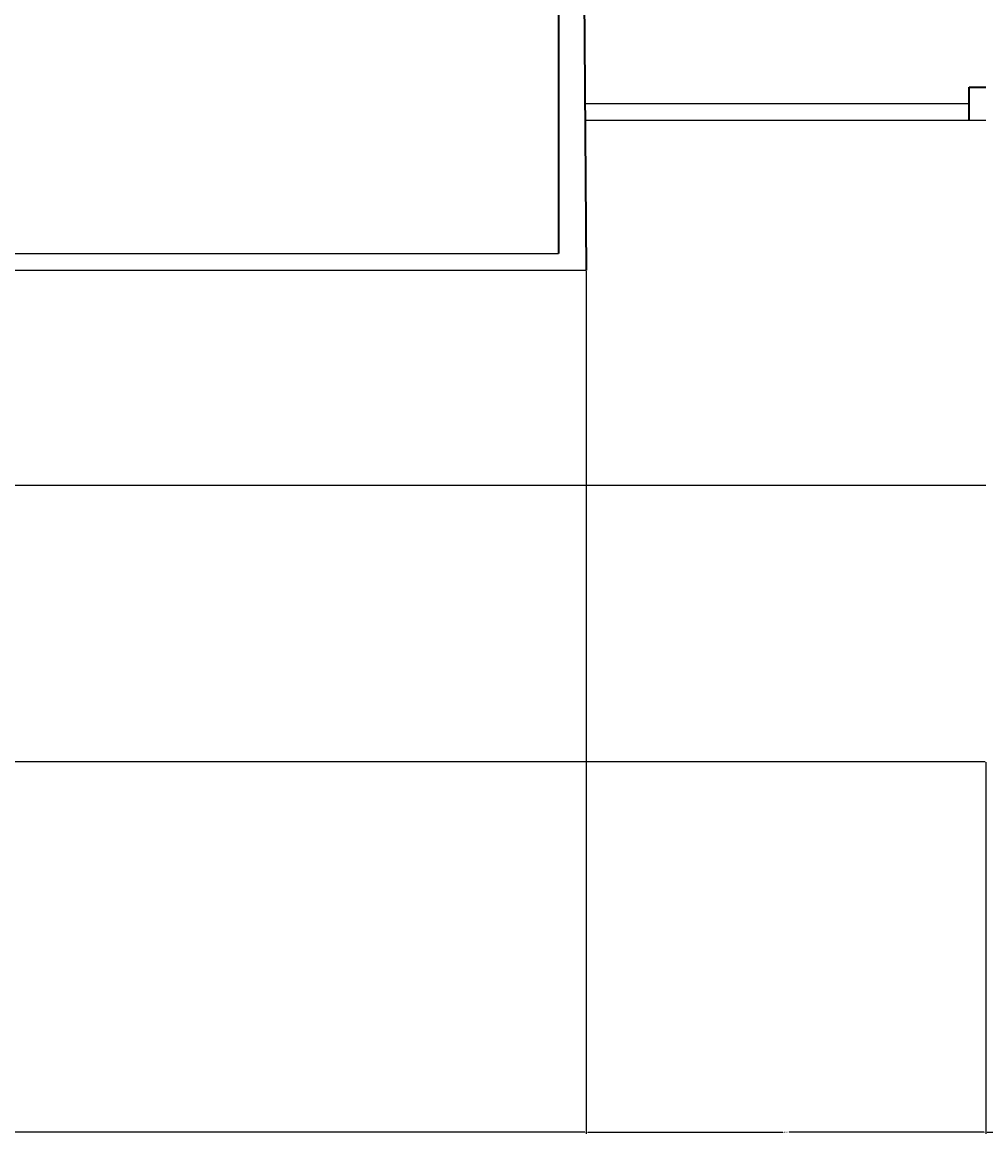
# Model space of a CAD drawing. Units: inches. Extents: x 1002 to 1561, y 1016 to 1994.
# Tile 2 of 8: x 1166 to 1282, y 1016 to 1149. Entities that reach past the tile are written whole.
import ezdxf

# ---------------------------------------------------------------- set-up
doc = ezdxf.new("R2010")
doc.units = ezdxf.units.IN
doc.header["$MEASUREMENT"] = 0
doc.layers.add('A-ANNO-DIMS', color=2, linetype='Continuous', lineweight=18)
doc.layers.add('A-WALL', color=7, linetype='Continuous', lineweight=35)
doc.layers.add('A-FLOR-EDGE', color=217, linetype='Continuous', lineweight=25, true_color=0x93278f)
doc.styles.get("Standard").update_dxf_attribs({"font": 'arial.ttf'})
doc.dimstyles.get("Standard").update_dxf_attribs({"dimtxt": 0.18, "dimasz": 0.18, "dimexe": 0.18, "dimexo": 0.0625, "dimgap": 0.09, "dimtad": 0, "dimtih": 1, "dimtoh": 1, "dimdec": 4, "dimzin": 0, "dimdsep": 46, "dimtxsty": 'Standard', "dimcen": 0.09, "dimadec": 0, "dimazin": 0, "dimtfac": 1, "dimtdec": 4, "dimtofl": 0, "dimtmove": 0, "dimatfit": 3, "dimfxl": 1, "dimtolj": 1, "dimtzin": 0, "dimarcsym": 0})

# ---------------------------------------------------------------- blocks, each defined once
blk = doc.blocks.new('*D16')
at = {"layer": 'A-ANNO-DIMS', "color": 0, "lineweight": -2, "transparency": 16777216}
for p, q in [((1046.37, 1119.51), (1001.74, 1119.51)), ((1001.92, 1119.33), (1001.92, 1090.18)), ((1001.92, 1060.67), (1001.92, 1089.82)), ((1281.73, 1060.49), (1001.74, 1060.49))]:
    blk.add_line(p, q, dxfattribs=at)
at = {"layer": 'A-ANNO-DIMS', "color": 0, "transparency": 16777216}
for points in [[(1001.89, 1119.33), (1001.95, 1119.33), (1001.92, 1119.51)], [(1001.89, 1060.67), (1001.95, 1060.67), (1001.92, 1060.49)]]:
    blk.add_solid(points, dxfattribs=at)
at = {"layer": 'Defpoints', "color": 0, "transparency": 16777216}
for p in [(1001.92, 1119.51), (1046.43, 1119.51), (1281.79, 1060.49)]:
    blk.add_point(p, dxfattribs=at)
at = {"layer": 'A-ANNO-DIMS', "color": 0, "transparency": 16777216, "insert": (1001.92, 1090), "char_height": 0.18, "attachment_point": 5}
blk.add_mtext('\\A1;59.02', dxfattribs=at)
blk = doc.blocks.new('*D17')
at = {"layer": 'A-ANNO-DIMS', "color": 0, "lineweight": -2, "transparency": 16777216}
for p, q in [((1233.77, 1119.45), (1233.77, 1015.8)), ((1046.43, 1093.59), (1046.43, 1015.8)), ((1046.61, 1015.98), (1139.65, 1015.98)), ((1233.59, 1015.98), (1140.56, 1015.98))]:
    blk.add_line(p, q, dxfattribs=at)
at = {"layer": 'A-ANNO-DIMS', "color": 0, "transparency": 16777216}
for points in [[(1046.61, 1016.01), (1046.61, 1015.95), (1046.43, 1015.98)], [(1233.59, 1016.01), (1233.59, 1015.95), (1233.77, 1015.98)]]:
    blk.add_solid(points, dxfattribs=at)
at = {"layer": 'Defpoints', "color": 0, "transparency": 16777216}
for p in [(1233.77, 1119.51), (1046.43, 1093.65), (1233.77, 1015.98)]:
    blk.add_point(p, dxfattribs=at)
at = {"layer": 'A-ANNO-DIMS', "color": 0, "transparency": 16777216, "insert": (1140.1, 1015.98), "char_height": 0.18, "attachment_point": 5}
blk.add_mtext('\\A1;187.34', dxfattribs=at)
blk = doc.blocks.new('*D18')
at = {"layer": 'A-ANNO-DIMS', "color": 0, "lineweight": -2, "transparency": 16777216}
for p, q in [((1233.77, 1119.45), (1233.77, 1015.8)), ((1281.79, 1060.43), (1281.79, 1015.8)), ((1233.95, 1015.98), (1257.39, 1015.98)), ((1281.61, 1015.98), (1258.18, 1015.98))]:
    blk.add_line(p, q, dxfattribs=at)
at = {"layer": 'A-ANNO-DIMS', "color": 0, "transparency": 16777216}
for points in [[(1233.95, 1016.01), (1233.95, 1015.95), (1233.77, 1015.98)], [(1281.61, 1016.01), (1281.61, 1015.95), (1281.79, 1015.98)]]:
    blk.add_solid(points, dxfattribs=at)
at = {"layer": 'Defpoints', "color": 0, "transparency": 16777216}
for p in [(1233.77, 1119.51), (1281.79, 1060.49), (1281.79, 1015.98)]:
    blk.add_point(p, dxfattribs=at)
at = {"layer": 'A-ANNO-DIMS', "color": 0, "transparency": 16777216, "insert": (1257.78, 1015.98), "char_height": 0.18, "attachment_point": 5}
blk.add_mtext('\\A1;48.02', dxfattribs=at)
blk = doc.blocks.new('*D19')
at = {"layer": 'A-ANNO-DIMS', "color": 0, "lineweight": -2, "transparency": 16777216}
for p, q in [((1413.43, 1141.45), (1413.43, 1015.8)), ((1281.79, 1060.43), (1281.79, 1015.8)), ((1281.97, 1015.98), (1347.16, 1015.98)), ((1413.25, 1015.98), (1348.07, 1015.98))]:
    blk.add_line(p, q, dxfattribs=at)
at = {"layer": 'A-ANNO-DIMS', "color": 0, "transparency": 16777216}
for points in [[(1281.97, 1016.01), (1281.97, 1015.95), (1281.79, 1015.98)], [(1413.25, 1016.01), (1413.25, 1015.95), (1413.43, 1015.98)]]:
    blk.add_solid(points, dxfattribs=at)
at = {"layer": 'Defpoints', "color": 0, "transparency": 16777216}
for p in [(1413.43, 1141.51), (1281.79, 1060.49), (1413.43, 1015.98)]:
    blk.add_point(p, dxfattribs=at)
at = {"layer": 'A-ANNO-DIMS', "color": 0, "transparency": 16777216, "insert": (1347.61, 1015.98), "char_height": 0.18, "attachment_point": 5}
blk.add_mtext('\\A1;131.64', dxfattribs=at)

msp = doc.modelspace()

# ---------------------------------------------------------------- linework, layer by layer
at = {"layer": 'A-FLOR-EDGE'}
for p, q in [((1279.793, 1139.51), (1233.649, 1139.51)), ((1281.793, 1137.51), (1233.649, 1137.51)), ((1050.434, 1121.51), (1230.434, 1121.51)), ((1233.759, 1121.51), (1233.773, 1121.51)), ((1046.434, 1119.51), (1233.773, 1119.51)), ((1281.793, 1093.652), (1046.434, 1093.652))]:
    msp.add_line(p, q, dxfattribs=at)
at = {"layer": 'A-WALL'}
for p, q in [((1230.434, 1168.702), (1230.434, 1121.51)), ((1233.434, 1168.702), (1233.773, 1119.51)), ((1279.793, 1141.51), (1281.793, 1141.51)), ((1279.793, 1137.51), (1279.793, 1141.51))]:
    msp.add_line(p, q, dxfattribs=at)

# ---------------------------------------------------------------- dimensions: what is measured, and where the dimension line sits
at = {"layer": 'A-ANNO-DIMS'}
for base, p1, p2, picture, middle in [((1413.434, 1015.98), (1281.793, 1060.49), (1413.434, 1141.51), '*D19', (1347.613, 1015.98)), ((1233.773, 1015.98), (1046.434, 1093.652), (1233.773, 1119.51), '*D17', (1140.103, 1015.98)), ((1281.793, 1015.98), (1233.773, 1119.51), (1281.793, 1060.49), '*D18', (1257.783, 1015.98))]:
    dim = msp.add_linear_dim(base=base, p1=p1, p2=p2, dimstyle='Standard', override={"dimdec": 2, "dimlfac": 1, "dimrnd": 0, "dimzin": 0, "dimdsep": 46, "dimlunit": 2}, dxfattribs=at)
    dim.commit()
    dim.dimension.update_dxf_attribs({"geometry": picture, "text_midpoint": middle})
dim = msp.add_linear_dim(base=(1001.924, 1119.51), p1=(1281.793, 1060.49), p2=(1046.434, 1119.51), angle=90, dimstyle='Standard', override={"dimdec": 2, "dimlfac": 1, "dimrnd": 0, "dimzin": 0, "dimdsep": 46, "dimlunit": 2}, dxfattribs=at)
dim.commit()
dim.dimension.update_dxf_attribs({"geometry": '*D16', "text_midpoint": (1001.924, 1090)})

doc.saveas('drawing.dxf')
